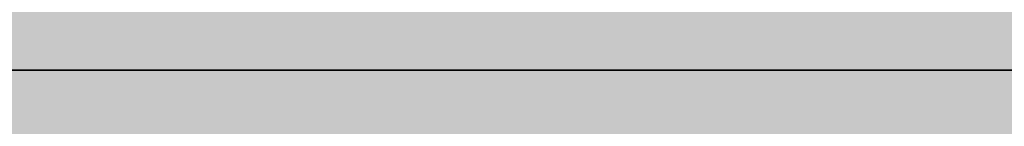
# Model space of a CAD drawing. Units: millimetres. Extents: x -22994 to 29398, y -19990 to 20176.
# Tile 76 of 135: x 226.355 to 227.437, y 84.498 to 84.615. Entities that reach past the tile are written whole.
import ezdxf
from ezdxf import colors
from ezdxf.entities.mleader import LeaderData, LeaderLine
from ezdxf.math import Vec2, Vec3

# ---------------------------------------------------------------- set-up
doc = ezdxf.new("R2010")
doc.units = ezdxf.units.MM
doc.header["$MEASUREMENT"] = 0
for name, color, linetype, lineweight in [('M-ANNO-TEXT', 7, 'Continuous', 25), ('M-DIMS', 2, 'Continuous', 18), ('M-EQPM-PATT', 7, 'Continuous', 18), ('M-PIPE', 7, 'Continuous', 35)]:
    doc.layers.add(name, color=color, linetype=linetype, lineweight=lineweight)
doc.styles.get("Standard").update_dxf_attribs({"font": 'arial.ttf'})
doc.dimstyles.get("Standard").update_dxf_attribs({"dimtxt": 0.18, "dimasz": 10000, "dimexe": 0.18, "dimexo": 0.0625, "dimgap": 0.09, "dimtad": 0, "dimtih": 1, "dimtoh": 1, "dimdec": 0, "dimzin": 0, "dimdsep": 46, "dimtxsty": 'Standard', "dimcen": 0.09, "dimadec": 0, "dimazin": 0, "dimtfac": 1, "dimtdec": 0, "dimtofl": 0, "dimtmove": 0, "dimatfit": 3, "dimfxl": 1, "dimtolj": 1, "dimtzin": 0, "dimlwd": 30, "dimarcsym": 0})

# ---------------------------------------------------------------- blocks, each defined once
blk = doc.blocks.new('*D2')
at = {"layer": 'Defpoints', "color": 0, "transparency": 16777216}
for p in [(6.6773, 10.2713), (290.852, 10.2713), (290.852, -5.0787)]:
    blk.add_point(p, dxfattribs=at)
at = {"layer": 'M-DIMS', "color": 0, "lineweight": -2, "transparency": 16777216}
for p, q in [((6.6773, 10.2088), (6.6773, -5.2587)), ((290.852, 10.2088), (290.852, -5.2587))]:
    blk.add_line(p, q, dxfattribs=at)
at = {"layer": 'M-DIMS', "color": 0, "lineweight": 30, "transparency": 16777216}
for p, q in [((-9993.3227, -5.0787), (-19993.3227, -5.0787)), ((10290.852, -5.0787), (20290.852, -5.0787))]:
    blk.add_line(p, q, dxfattribs=at)
at = {"layer": 'M-DIMS', "color": 0, "transparency": 16777216}
for points in [[(-9993.3227, 1661.5879), (-9993.3227, -1671.7454), (6.6773, -5.0787)], [(10290.852, 1661.5879), (10290.852, -1671.7454), (290.852, -5.0787)]]:
    blk.add_solid(points, dxfattribs=at)
at = {"layer": 'M-DIMS', "color": 0, "transparency": 16777216, "insert": (148.7647, -5.0787), "char_height": 0.18, "attachment_point": 5}
blk.add_mtext('\\A1;284.2', dxfattribs=at)
blk = doc.blocks.new('*D3')
at = {"layer": 'Defpoints', "color": 0, "transparency": 16777216}
for p in [(110.2647, 204.1654), (110.2647, 176.3662), (95.8327, 127.967)]:
    blk.add_point(p, dxfattribs=at)
at = {"layer": 'M-DIMS', "color": 0, "lineweight": -2, "transparency": 16777216}
for p, q in [((95.8327, 128.0295), (95.8327, 204.3454)), ((110.2647, 176.4287), (110.2647, 204.3454))]:
    blk.add_line(p, q, dxfattribs=at)
at = {"layer": 'M-DIMS', "color": 0, "lineweight": 30, "transparency": 16777216}
for p, q in [((-9904.1673, 204.1654), (-19904.1673, 204.1654)), ((10110.2647, 204.1654), (20110.2647, 204.1654))]:
    blk.add_line(p, q, dxfattribs=at)
at = {"layer": 'M-DIMS', "color": 0, "transparency": 16777216}
for points in [[(-9904.1673, 1870.8321), (-9904.1673, -1462.5013), (95.8327, 204.1654)], [(10110.2647, 1870.8321), (10110.2647, -1462.5013), (110.2647, 204.1654)]]:
    blk.add_solid(points, dxfattribs=at)
at = {"layer": 'M-DIMS', "color": 0, "transparency": 16777216, "insert": (103.0487, 204.1654), "char_height": 0.18, "attachment_point": 5}
blk.add_mtext('\\A1;14.432', dxfattribs=at)
blk = doc.blocks.new('*D4')
at = {"layer": 'Defpoints', "color": 0, "transparency": 16777216}
for p in [(116.2647, 204.1654), (110.2647, 176.3662), (116.2647, 176.3662)]:
    blk.add_point(p, dxfattribs=at)
at = {"layer": 'M-DIMS', "color": 0, "lineweight": -2, "transparency": 16777216}
for p, q in [((110.2647, 176.4287), (110.2647, 204.3454)), ((116.2647, 176.4287), (116.2647, 204.3454))]:
    blk.add_line(p, q, dxfattribs=at)
at = {"layer": 'M-DIMS', "color": 0, "lineweight": 30, "transparency": 16777216}
for p, q in [((-9889.7353, 204.1654), (-19889.7353, 204.1654)), ((10116.2647, 204.1654), (20116.2647, 204.1654))]:
    blk.add_line(p, q, dxfattribs=at)
at = {"layer": 'M-DIMS', "color": 0, "transparency": 16777216}
for points in [[(-9889.7353, 1870.8321), (-9889.7353, -1462.5013), (110.2647, 204.1654)], [(10116.2647, 1870.8321), (10116.2647, -1462.5013), (116.2647, 204.1654)]]:
    blk.add_solid(points, dxfattribs=at)
at = {"layer": 'M-DIMS', "color": 0, "transparency": 16777216, "insert": (113.2647, 204.1654), "char_height": 0.18, "attachment_point": 5}
blk.add_mtext('\\A1;6', dxfattribs=at)
blk = doc.blocks.new('*D5')
at = {"layer": 'Defpoints', "color": 0, "transparency": 16777216}
for p in [(181.2647, 204.1654), (116.2647, 176.3662), (181.2647, 176.3662)]:
    blk.add_point(p, dxfattribs=at)
at = {"layer": 'M-DIMS', "color": 0, "lineweight": -2, "transparency": 16777216}
for p, q in [((116.2647, 176.4287), (116.2647, 204.3454)), ((181.2647, 176.4287), (181.2647, 204.3454))]:
    blk.add_line(p, q, dxfattribs=at)
at = {"layer": 'M-DIMS', "color": 0, "lineweight": 30, "transparency": 16777216}
for p, q in [((-9883.7353, 204.1654), (-19883.7353, 204.1654)), ((10181.2647, 204.1654), (20181.2647, 204.1654))]:
    blk.add_line(p, q, dxfattribs=at)
at = {"layer": 'M-DIMS', "color": 0, "transparency": 16777216}
for points in [[(-9883.7353, 1870.8321), (-9883.7353, -1462.5013), (116.2647, 204.1654)], [(10181.2647, 1870.8321), (10181.2647, -1462.5013), (181.2647, 204.1654)]]:
    blk.add_solid(points, dxfattribs=at)
at = {"layer": 'M-DIMS', "color": 0, "transparency": 16777216, "insert": (148.7647, 204.1654), "char_height": 0.18, "attachment_point": 5}
blk.add_mtext('\\A1;65', dxfattribs=at)
blk = doc.blocks.new('*D6')
at = {"layer": 'Defpoints', "color": 0, "transparency": 16777216}
for p in [(187.2647, 204.1654), (181.2647, 176.3662), (187.2647, 176.3662)]:
    blk.add_point(p, dxfattribs=at)
at = {"layer": 'M-DIMS', "color": 0, "lineweight": -2, "transparency": 16777216}
for p, q in [((181.2647, 176.4287), (181.2647, 204.3454)), ((187.2647, 176.4287), (187.2647, 204.3454))]:
    blk.add_line(p, q, dxfattribs=at)
at = {"layer": 'M-DIMS', "color": 0, "lineweight": 30, "transparency": 16777216}
for p, q in [((-9818.7353, 204.1654), (-19818.7353, 204.1654)), ((10187.2647, 204.1654), (20187.2647, 204.1654))]:
    blk.add_line(p, q, dxfattribs=at)
at = {"layer": 'M-DIMS', "color": 0, "transparency": 16777216}
for points in [[(-9818.7353, 1870.8321), (-9818.7353, -1462.5013), (181.2647, 204.1654)], [(10187.2647, 1870.8321), (10187.2647, -1462.5013), (187.2647, 204.1654)]]:
    blk.add_solid(points, dxfattribs=at)
at = {"layer": 'M-DIMS', "color": 0, "transparency": 16777216, "insert": (184.2647, 204.1654), "char_height": 0.18, "attachment_point": 5}
blk.add_mtext('\\A1;6', dxfattribs=at)
blk = doc.blocks.new('*D7')
at = {"layer": 'Defpoints', "color": 0, "transparency": 16777216}
for p in [(201.6967, 204.1654), (187.2647, 176.3662), (201.6967, 127.967)]:
    blk.add_point(p, dxfattribs=at)
at = {"layer": 'M-DIMS', "color": 0, "lineweight": -2, "transparency": 16777216}
for p, q in [((187.2647, 176.4287), (187.2647, 204.3454)), ((201.6967, 128.0295), (201.6967, 204.3454))]:
    blk.add_line(p, q, dxfattribs=at)
at = {"layer": 'M-DIMS', "color": 0, "lineweight": 30, "transparency": 16777216}
for p, q in [((-9812.7353, 204.1654), (-19812.7353, 204.1654)), ((10201.6967, 204.1654), (20201.6967, 204.1654))]:
    blk.add_line(p, q, dxfattribs=at)
at = {"layer": 'M-DIMS', "color": 0, "transparency": 16777216}
for points in [[(-9812.7353, 1870.8321), (-9812.7353, -1462.5013), (187.2647, 204.1654)], [(10201.6967, 1870.8321), (10201.6967, -1462.5013), (201.6967, 204.1654)]]:
    blk.add_solid(points, dxfattribs=at)
at = {"layer": 'M-DIMS', "color": 0, "transparency": 16777216, "insert": (194.4807, 204.1654), "char_height": 0.18, "attachment_point": 5}
blk.add_mtext('\\A1;14.432', dxfattribs=at)
blk = doc.blocks.new('*D8')
at = {"layer": 'Defpoints', "color": 0, "transparency": 16777216}
for p in [(227.6485, 204.1654), (227.6485, 146.7296), (201.6967, 127.967)]:
    blk.add_point(p, dxfattribs=at)
at = {"layer": 'M-DIMS', "color": 0, "lineweight": -2, "transparency": 16777216}
for p, q in [((201.6967, 128.0295), (201.6967, 204.3454)), ((227.6485, 146.7921), (227.6485, 204.3454))]:
    blk.add_line(p, q, dxfattribs=at)
at = {"layer": 'M-DIMS', "color": 0, "lineweight": 30, "transparency": 16777216}
for p, q in [((-9798.3033, 204.1654), (-19798.3033, 204.1654)), ((10227.6485, 204.1654), (20227.6485, 204.1654))]:
    blk.add_line(p, q, dxfattribs=at)
at = {"layer": 'M-DIMS', "color": 0, "transparency": 16777216}
for points in [[(-9798.3033, 1870.8321), (-9798.3033, -1462.5013), (201.6967, 204.1654)], [(10227.6485, 1870.8321), (10227.6485, -1462.5013), (227.6485, 204.1654)]]:
    blk.add_solid(points, dxfattribs=at)
at = {"layer": 'M-DIMS', "color": 0, "transparency": 16777216, "insert": (214.6726, 204.1654), "char_height": 0.18, "attachment_point": 5}
blk.add_mtext('\\A1;25.95', dxfattribs=at)
blk = doc.blocks.new('*D9')
at = {"layer": 'Defpoints', "color": 0, "transparency": 16777216}
for p in [(187.2647, 176.3662), (306.202, 176.3662), (290.852, 10.2713)]:
    blk.add_point(p, dxfattribs=at)
at = {"layer": 'M-DIMS', "color": 0, "lineweight": 30, "transparency": 16777216}
for p, q in [((306.202, 10176.3662), (306.202, 20176.3662)), ((306.202, -9989.7287), (306.202, -19989.7287))]:
    blk.add_line(p, q, dxfattribs=at)
at = {"layer": 'M-DIMS', "color": 0, "lineweight": -2, "transparency": 16777216}
for p, q in [((187.3272, 176.3662), (306.382, 176.3662)), ((290.9145, 10.2713), (306.382, 10.2713))]:
    blk.add_line(p, q, dxfattribs=at)
at = {"layer": 'M-DIMS', "color": 0, "transparency": 16777216}
for points in [[(-1360.4646, 10176.3662), (1972.8687, 10176.3662), (306.202, 176.3662)], [(-1360.4646, -9989.7287), (1972.8687, -9989.7287), (306.202, 10.2713)]]:
    blk.add_solid(points, dxfattribs=at)
at = {"layer": 'M-DIMS', "color": 0, "transparency": 16777216, "insert": (306.202, 93.3187), "char_height": 0.18, "attachment_point": 5}
blk.add_mtext('\\A1;166.1', dxfattribs=at)
blk = doc.blocks.new('*D10')
at = {"layer": 'Defpoints', "color": 0, "transparency": 16777216}
for p in [(125.6498, 136.0713), (133.3459, 136.0713), (133.3459, -5.0787)]:
    blk.add_point(p, dxfattribs=at)
at = {"layer": 'M-DIMS', "color": 0, "lineweight": -2, "transparency": 16777216}
for p, q in [((125.6498, 136.0088), (125.6498, -5.2587)), ((133.3459, 136.0088), (133.3459, -5.2587))]:
    blk.add_line(p, q, dxfattribs=at)
at = {"layer": 'M-DIMS', "color": 0, "lineweight": 30, "transparency": 16777216}
for p, q in [((-9874.3502, -5.0787), (-19874.3502, -5.0787)), ((10133.3459, -5.0787), (20133.3459, -5.0787))]:
    blk.add_line(p, q, dxfattribs=at)
at = {"layer": 'M-DIMS', "color": 0, "transparency": 16777216}
for points in [[(-9874.3502, 1661.5879), (-9874.3502, -1671.7454), (125.6498, -5.0787)], [(10133.3459, 1661.5879), (10133.3459, -1671.7454), (133.3459, -5.0787)]]:
    blk.add_solid(points, dxfattribs=at)
at = {"layer": 'M-DIMS', "color": 0, "transparency": 16777216, "insert": (129.4978, -5.0787), "char_height": 0.18, "attachment_point": 5}
blk.add_mtext('\\A1;7.696', dxfattribs=at)
blk = doc.blocks.new('*D11')
at = {"layer": 'Defpoints', "color": 0, "transparency": 16777216}
for p in [(133.3459, 136.0713), (135.6498, 136.0713), (135.6498, -5.0787)]:
    blk.add_point(p, dxfattribs=at)
at = {"layer": 'M-DIMS', "color": 0, "lineweight": -2, "transparency": 16777216}
for p, q in [((133.3459, 136.0088), (133.3459, -5.2587)), ((135.6498, 136.0088), (135.6498, -5.2587))]:
    blk.add_line(p, q, dxfattribs=at)
at = {"layer": 'M-DIMS', "color": 0, "lineweight": 30, "transparency": 16777216}
for p, q in [((-9866.6541, -5.0787), (-19866.6541, -5.0787)), ((10135.6498, -5.0787), (20135.6498, -5.0787))]:
    blk.add_line(p, q, dxfattribs=at)
at = {"layer": 'M-DIMS', "color": 0, "transparency": 16777216}
for points in [[(-9866.6541, 1661.5879), (-9866.6541, -1671.7454), (133.3459, -5.0787)], [(10135.6498, 1661.5879), (10135.6498, -1671.7454), (135.6498, -5.0787)]]:
    blk.add_solid(points, dxfattribs=at)
at = {"layer": 'M-DIMS', "color": 0, "transparency": 16777216, "insert": (134.4978, -5.0787), "char_height": 0.18, "attachment_point": 5}
blk.add_mtext('\\A1;2.304', dxfattribs=at)
blk = doc.blocks.new('*D12')
at = {"layer": 'Defpoints', "color": 0, "transparency": 16777216}
for p in [(135.6498, 136.0713), (145.6498, 136.0713), (145.6498, -5.0787)]:
    blk.add_point(p, dxfattribs=at)
at = {"layer": 'M-DIMS', "color": 0, "lineweight": -2, "transparency": 16777216}
for p, q in [((135.6498, 136.0088), (135.6498, -5.2587)), ((145.6498, 136.0088), (145.6498, -5.2587))]:
    blk.add_line(p, q, dxfattribs=at)
at = {"layer": 'M-DIMS', "color": 0, "lineweight": 30, "transparency": 16777216}
for p, q in [((-9864.3502, -5.0787), (-19864.3502, -5.0787)), ((10145.6498, -5.0787), (20145.6498, -5.0787))]:
    blk.add_line(p, q, dxfattribs=at)
at = {"layer": 'M-DIMS', "color": 0, "transparency": 16777216}
for points in [[(-9864.3502, 1661.5879), (-9864.3502, -1671.7454), (135.6498, -5.0787)], [(10145.6498, 1661.5879), (10145.6498, -1671.7454), (145.6498, -5.0787)]]:
    blk.add_solid(points, dxfattribs=at)
at = {"layer": 'M-DIMS', "color": 0, "transparency": 16777216, "insert": (140.6498, -5.0787), "char_height": 0.18, "attachment_point": 5}
blk.add_mtext('\\A1;10', dxfattribs=at)
blk = doc.blocks.new('*D13')
at = {"layer": 'Defpoints', "color": 0, "transparency": 16777216}
for p in [(145.6498, 136.0713), (155.6498, 136.0713), (155.6498, -5.0787)]:
    blk.add_point(p, dxfattribs=at)
at = {"layer": 'M-DIMS', "color": 0, "lineweight": -2, "transparency": 16777216}
for p, q in [((145.6498, 136.0088), (145.6498, -5.2587)), ((155.6498, 136.0088), (155.6498, -5.2587))]:
    blk.add_line(p, q, dxfattribs=at)
at = {"layer": 'M-DIMS', "color": 0, "lineweight": 30, "transparency": 16777216}
for p, q in [((-9854.3502, -5.0787), (-19854.3502, -5.0787)), ((10155.6498, -5.0787), (20155.6498, -5.0787))]:
    blk.add_line(p, q, dxfattribs=at)
at = {"layer": 'M-DIMS', "color": 0, "transparency": 16777216}
for points in [[(-9854.3502, 1661.5879), (-9854.3502, -1671.7454), (145.6498, -5.0787)], [(10155.6498, 1661.5879), (10155.6498, -1671.7454), (155.6498, -5.0787)]]:
    blk.add_solid(points, dxfattribs=at)
at = {"layer": 'M-DIMS', "color": 0, "transparency": 16777216, "insert": (150.6498, -5.0787), "char_height": 0.18, "attachment_point": 5}
blk.add_mtext('\\A1;10', dxfattribs=at)
blk = doc.blocks.new('*D14')
at = {"layer": 'Defpoints', "color": 0, "transparency": 16777216}
for p in [(155.6498, 136.0713), (165.6498, 136.0713), (165.6498, -5.0787)]:
    blk.add_point(p, dxfattribs=at)
at = {"layer": 'M-DIMS', "color": 0, "lineweight": -2, "transparency": 16777216}
for p, q in [((155.6498, 136.0088), (155.6498, -5.2587)), ((165.6498, 136.0088), (165.6498, -5.2587))]:
    blk.add_line(p, q, dxfattribs=at)
at = {"layer": 'M-DIMS', "color": 0, "lineweight": 30, "transparency": 16777216}
for p, q in [((-9844.3502, -5.0787), (-19844.3502, -5.0787)), ((10165.6498, -5.0787), (20165.6498, -5.0787))]:
    blk.add_line(p, q, dxfattribs=at)
at = {"layer": 'M-DIMS', "color": 0, "transparency": 16777216}
for points in [[(-9844.3502, 1661.5879), (-9844.3502, -1671.7454), (155.6498, -5.0787)], [(10165.6498, 1661.5879), (10165.6498, -1671.7454), (165.6498, -5.0787)]]:
    blk.add_solid(points, dxfattribs=at)
at = {"layer": 'M-DIMS', "color": 0, "transparency": 16777216, "insert": (160.6498, -5.0787), "char_height": 0.18, "attachment_point": 5}
blk.add_mtext('\\A1;10', dxfattribs=at)
blk = doc.blocks.new('*D15')
at = {"layer": 'Defpoints', "color": 0, "transparency": 16777216}
for p in [(173.3459, 154.788), (173.3459, 136.0713), (306.202, 136.0713)]:
    blk.add_point(p, dxfattribs=at)
at = {"layer": 'M-DIMS', "color": 0, "lineweight": 30, "transparency": 16777216}
for p, q in [((306.202, 10154.788), (306.202, 20154.788)), ((306.202, -9863.9287), (306.202, -19863.9287))]:
    blk.add_line(p, q, dxfattribs=at)
at = {"layer": 'M-DIMS', "color": 0, "lineweight": -2, "transparency": 16777216}
for p, q in [((173.4084, 154.788), (306.382, 154.788)), ((173.4084, 136.0713), (306.382, 136.0713))]:
    blk.add_line(p, q, dxfattribs=at)
at = {"layer": 'M-DIMS', "color": 0, "transparency": 16777216}
for points in [[(-1360.4646, 10154.788), (1972.8687, 10154.788), (306.202, 154.788)], [(-1360.4646, -9863.9287), (1972.8687, -9863.9287), (306.202, 136.0713)]]:
    blk.add_solid(points, dxfattribs=at)
at = {"layer": 'M-DIMS', "color": 0, "transparency": 16777216, "insert": (306.202, 145.4297), "char_height": 0.18, "attachment_point": 5}
blk.add_mtext('\\A1;18.717', dxfattribs=at)
blk = doc.blocks.new('*D16')
at = {"layer": 'Defpoints', "color": 0, "transparency": 16777216}
for p in [(120.1702, 204.1654), (110.4658, 48.0349), (120.1702, 48.0349)]:
    blk.add_point(p, dxfattribs=at)
at = {"layer": 'M-DIMS', "color": 0, "lineweight": -2, "transparency": 16777216}
for p, q in [((110.4658, 48.0974), (110.4658, 204.3454)), ((120.1702, 48.0974), (120.1702, 204.3454))]:
    blk.add_line(p, q, dxfattribs=at)
at = {"layer": 'M-DIMS', "color": 0, "lineweight": 30, "transparency": 16777216}
for p, q in [((-9889.5342, 204.1654), (-19889.5342, 204.1654)), ((10120.1702, 204.1654), (20120.1702, 204.1654))]:
    blk.add_line(p, q, dxfattribs=at)
at = {"layer": 'M-DIMS', "color": 0, "transparency": 16777216}
for points in [[(-9889.5342, 1870.8321), (-9889.5342, -1462.5013), (110.4658, 204.1654)], [(10120.1702, 1870.8321), (10120.1702, -1462.5013), (120.1702, 204.1654)]]:
    blk.add_solid(points, dxfattribs=at)
at = {"layer": 'M-DIMS', "color": 0, "transparency": 16777216, "insert": (115.318, 204.1654), "char_height": 0.18, "attachment_point": 5}
blk.add_mtext('\\A1;9.704', dxfattribs=at)
blk = doc.blocks.new('*D17')
at = {"layer": 'Defpoints', "color": 0, "transparency": 16777216}
for p in [(126.1702, 204.1654), (120.1702, 48.0349), (126.1702, 48.0349)]:
    blk.add_point(p, dxfattribs=at)
at = {"layer": 'M-DIMS', "color": 0, "lineweight": -2, "transparency": 16777216}
for p, q in [((120.1702, 48.0974), (120.1702, 204.3454)), ((126.1702, 48.0974), (126.1702, 204.3454))]:
    blk.add_line(p, q, dxfattribs=at)
at = {"layer": 'M-DIMS', "color": 0, "lineweight": 30, "transparency": 16777216}
for p, q in [((-9879.8298, 204.1654), (-19879.8298, 204.1654)), ((10126.1702, 204.1654), (20126.1702, 204.1654))]:
    blk.add_line(p, q, dxfattribs=at)
at = {"layer": 'M-DIMS', "color": 0, "transparency": 16777216}
for points in [[(-9879.8298, 1870.8321), (-9879.8298, -1462.5013), (120.1702, 204.1654)], [(10126.1702, 1870.8321), (10126.1702, -1462.5013), (126.1702, 204.1654)]]:
    blk.add_solid(points, dxfattribs=at)
at = {"layer": 'M-DIMS', "color": 0, "transparency": 16777216, "insert": (123.1702, 204.1654), "char_height": 0.18, "attachment_point": 5}
blk.add_mtext('\\A1;6', dxfattribs=at)
blk = doc.blocks.new('*D18')
at = {"layer": 'Defpoints', "color": 0, "transparency": 16777216}
for p in [(132.1702, 204.1654), (126.1702, 48.0349), (132.1702, 48.0349)]:
    blk.add_point(p, dxfattribs=at)
at = {"layer": 'M-DIMS', "color": 0, "lineweight": -2, "transparency": 16777216}
for p, q in [((126.1702, 48.0974), (126.1702, 204.3454)), ((132.1702, 48.0974), (132.1702, 204.3454))]:
    blk.add_line(p, q, dxfattribs=at)
at = {"layer": 'M-DIMS', "color": 0, "lineweight": 30, "transparency": 16777216}
for p, q in [((-9873.8298, 204.1654), (-19873.8298, 204.1654)), ((10132.1702, 204.1654), (20132.1702, 204.1654))]:
    blk.add_line(p, q, dxfattribs=at)
at = {"layer": 'M-DIMS', "color": 0, "transparency": 16777216}
for points in [[(-9873.8298, 1870.8321), (-9873.8298, -1462.5013), (126.1702, 204.1654)], [(10132.1702, 1870.8321), (10132.1702, -1462.5013), (132.1702, 204.1654)]]:
    blk.add_solid(points, dxfattribs=at)
at = {"layer": 'M-DIMS', "color": 0, "transparency": 16777216, "insert": (129.1702, 204.1654), "char_height": 0.18, "attachment_point": 5}
blk.add_mtext('\\A1;6', dxfattribs=at)
blk = doc.blocks.new('*D19')
at = {"layer": 'Defpoints', "color": 0, "transparency": 16777216}
for p in [(138.1702, 204.1654), (132.1702, 48.0349), (138.1702, 48.0349)]:
    blk.add_point(p, dxfattribs=at)
at = {"layer": 'M-DIMS', "color": 0, "lineweight": -2, "transparency": 16777216}
for p, q in [((132.1702, 48.0974), (132.1702, 204.3454)), ((138.1702, 48.0974), (138.1702, 204.3454))]:
    blk.add_line(p, q, dxfattribs=at)
at = {"layer": 'M-DIMS', "color": 0, "lineweight": 30, "transparency": 16777216}
for p, q in [((-9867.8298, 204.1654), (-19867.8298, 204.1654)), ((10138.1702, 204.1654), (20138.1702, 204.1654))]:
    blk.add_line(p, q, dxfattribs=at)
at = {"layer": 'M-DIMS', "color": 0, "transparency": 16777216}
for points in [[(-9867.8298, 1870.8321), (-9867.8298, -1462.5013), (132.1702, 204.1654)], [(10138.1702, 1870.8321), (10138.1702, -1462.5013), (138.1702, 204.1654)]]:
    blk.add_solid(points, dxfattribs=at)
at = {"layer": 'M-DIMS', "color": 0, "transparency": 16777216, "insert": (135.1702, 204.1654), "char_height": 0.18, "attachment_point": 5}
blk.add_mtext('\\A1;6', dxfattribs=at)
blk = doc.blocks.new('*D20')
at = {"layer": 'Defpoints', "color": 0, "transparency": 16777216}
for p in [(144.1702, 204.1654), (138.1702, 48.0349), (144.1702, 48.0349)]:
    blk.add_point(p, dxfattribs=at)
at = {"layer": 'M-DIMS', "color": 0, "lineweight": -2, "transparency": 16777216}
for p, q in [((138.1702, 48.0974), (138.1702, 204.3454)), ((144.1702, 48.0974), (144.1702, 204.3454))]:
    blk.add_line(p, q, dxfattribs=at)
at = {"layer": 'M-DIMS', "color": 0, "lineweight": 30, "transparency": 16777216}
for p, q in [((-9861.8298, 204.1654), (-19861.8298, 204.1654)), ((10144.1702, 204.1654), (20144.1702, 204.1654))]:
    blk.add_line(p, q, dxfattribs=at)
at = {"layer": 'M-DIMS', "color": 0, "transparency": 16777216}
for points in [[(-9861.8298, 1870.8321), (-9861.8298, -1462.5013), (138.1702, 204.1654)], [(10144.1702, 1870.8321), (10144.1702, -1462.5013), (144.1702, 204.1654)]]:
    blk.add_solid(points, dxfattribs=at)
at = {"layer": 'M-DIMS', "color": 0, "transparency": 16777216, "insert": (141.1702, 204.1654), "char_height": 0.18, "attachment_point": 5}
blk.add_mtext('\\A1;6', dxfattribs=at)
blk = doc.blocks.new('*D21')
at = {"layer": 'Defpoints', "color": 0, "transparency": 16777216}
for p in [(149.1157, 204.1654), (144.1702, 48.0349), (149.1157, 48.0349)]:
    blk.add_point(p, dxfattribs=at)
at = {"layer": 'M-DIMS', "color": 0, "lineweight": -2, "transparency": 16777216}
for p, q in [((144.1702, 48.0974), (144.1702, 204.3454)), ((149.1157, 48.0974), (149.1157, 204.3454))]:
    blk.add_line(p, q, dxfattribs=at)
at = {"layer": 'M-DIMS', "color": 0, "lineweight": 30, "transparency": 16777216}
for p, q in [((-9855.8298, 204.1654), (-19855.8298, 204.1654)), ((10149.1157, 204.1654), (20149.1157, 204.1654))]:
    blk.add_line(p, q, dxfattribs=at)
at = {"layer": 'M-DIMS', "color": 0, "transparency": 16777216}
for points in [[(-9855.8298, 1870.8321), (-9855.8298, -1462.5013), (144.1702, 204.1654)], [(10149.1157, 1870.8321), (10149.1157, -1462.5013), (149.1157, 204.1654)]]:
    blk.add_solid(points, dxfattribs=at)
at = {"layer": 'M-DIMS', "color": 0, "transparency": 16777216, "insert": (146.6429, 204.1654), "char_height": 0.18, "attachment_point": 5}
blk.add_mtext('\\A1;4.945', dxfattribs=at)
blk = doc.blocks.new('*D22')
at = {"layer": 'Defpoints', "color": 0, "transparency": 16777216}
for p in [(149.1157, 30.9895), (155.1157, 30.9895), (155.1157, -5.0787)]:
    blk.add_point(p, dxfattribs=at)
at = {"layer": 'M-DIMS', "color": 0, "lineweight": -2, "transparency": 16777216}
for p, q in [((149.1157, 30.927), (149.1157, -5.2587)), ((155.1157, 30.927), (155.1157, -5.2587))]:
    blk.add_line(p, q, dxfattribs=at)
at = {"layer": 'M-DIMS', "color": 0, "lineweight": 30, "transparency": 16777216}
for p, q in [((-9850.8843, -5.0787), (-19850.8843, -5.0787)), ((10155.1157, -5.0787), (20155.1157, -5.0787))]:
    blk.add_line(p, q, dxfattribs=at)
at = {"layer": 'M-DIMS', "color": 0, "transparency": 16777216}
for points in [[(-9850.8843, 1661.5879), (-9850.8843, -1671.7454), (149.1157, -5.0787)], [(10155.1157, 1661.5879), (10155.1157, -1671.7454), (155.1157, -5.0787)]]:
    blk.add_solid(points, dxfattribs=at)
at = {"layer": 'M-DIMS', "color": 0, "transparency": 16777216, "insert": (152.1157, -5.0787), "char_height": 0.18, "attachment_point": 5}
blk.add_mtext('\\A1;6', dxfattribs=at)
blk = doc.blocks.new('*D23')
at = {"layer": 'Defpoints', "color": 0, "transparency": 16777216}
for p in [(155.1157, 30.9895), (161.1157, 30.9895), (161.1157, -5.0787)]:
    blk.add_point(p, dxfattribs=at)
at = {"layer": 'M-DIMS', "color": 0, "lineweight": -2, "transparency": 16777216}
for p, q in [((155.1157, 30.927), (155.1157, -5.2587)), ((161.1157, 30.927), (161.1157, -5.2587))]:
    blk.add_line(p, q, dxfattribs=at)
at = {"layer": 'M-DIMS', "color": 0, "lineweight": 30, "transparency": 16777216}
for p, q in [((-9844.8843, -5.0787), (-19844.8843, -5.0787)), ((10161.1157, -5.0787), (20161.1157, -5.0787))]:
    blk.add_line(p, q, dxfattribs=at)
at = {"layer": 'M-DIMS', "color": 0, "transparency": 16777216}
for points in [[(-9844.8843, 1661.5879), (-9844.8843, -1671.7454), (155.1157, -5.0787)], [(10161.1157, 1661.5879), (10161.1157, -1671.7454), (161.1157, -5.0787)]]:
    blk.add_solid(points, dxfattribs=at)
at = {"layer": 'M-DIMS', "color": 0, "transparency": 16777216, "insert": (158.1157, -5.0787), "char_height": 0.18, "attachment_point": 5}
blk.add_mtext('\\A1;6', dxfattribs=at)
blk = doc.blocks.new('*D24')
at = {"layer": 'Defpoints', "color": 0, "transparency": 16777216}
for p in [(161.1157, 30.9895), (166.4387, 30.9895), (166.4387, -5.0787)]:
    blk.add_point(p, dxfattribs=at)
at = {"layer": 'M-DIMS', "color": 0, "lineweight": -2, "transparency": 16777216}
for p, q in [((161.1157, 30.927), (161.1157, -5.2587)), ((166.4387, 30.927), (166.4387, -5.2587))]:
    blk.add_line(p, q, dxfattribs=at)
at = {"layer": 'M-DIMS', "color": 0, "lineweight": 30, "transparency": 16777216}
for p, q in [((-9838.8843, -5.0787), (-19838.8843, -5.0787)), ((10166.4387, -5.0787), (20166.4387, -5.0787))]:
    blk.add_line(p, q, dxfattribs=at)
at = {"layer": 'M-DIMS', "color": 0, "transparency": 16777216}
for points in [[(-9838.8843, 1661.5879), (-9838.8843, -1671.7454), (161.1157, -5.0787)], [(10166.4387, 1661.5879), (10166.4387, -1671.7454), (166.4387, -5.0787)]]:
    blk.add_solid(points, dxfattribs=at)
at = {"layer": 'M-DIMS', "color": 0, "transparency": 16777216, "insert": (163.7772, -5.0787), "char_height": 0.18, "attachment_point": 5}
blk.add_mtext('\\A1;5.323', dxfattribs=at)
blk = doc.blocks.new('*D25')
at = {"layer": 'Defpoints', "color": 0, "transparency": 16777216}
for p in [(166.4387, 30.9895), (172.4387, 30.9895), (172.4387, -5.0787)]:
    blk.add_point(p, dxfattribs=at)
at = {"layer": 'M-DIMS', "color": 0, "lineweight": -2, "transparency": 16777216}
for p, q in [((166.4387, 30.927), (166.4387, -5.2587)), ((172.4387, 30.927), (172.4387, -5.2587))]:
    blk.add_line(p, q, dxfattribs=at)
at = {"layer": 'M-DIMS', "color": 0, "lineweight": 30, "transparency": 16777216}
for p, q in [((-9833.5613, -5.0787), (-19833.5613, -5.0787)), ((10172.4387, -5.0787), (20172.4387, -5.0787))]:
    blk.add_line(p, q, dxfattribs=at)
at = {"layer": 'M-DIMS', "color": 0, "transparency": 16777216}
for points in [[(-9833.5613, 1661.5879), (-9833.5613, -1671.7454), (166.4387, -5.0787)], [(10172.4387, 1661.5879), (10172.4387, -1671.7454), (172.4387, -5.0787)]]:
    blk.add_solid(points, dxfattribs=at)
at = {"layer": 'M-DIMS', "color": 0, "transparency": 16777216, "insert": (169.4387, -5.0787), "char_height": 0.18, "attachment_point": 5}
blk.add_mtext('\\A1;6', dxfattribs=at)
blk = doc.blocks.new('*D26')
at = {"layer": 'Defpoints', "color": 0, "transparency": 16777216}
for p in [(172.4387, 30.9895), (178.4387, 30.9895), (178.4387, -5.0787)]:
    blk.add_point(p, dxfattribs=at)
at = {"layer": 'M-DIMS', "color": 0, "lineweight": -2, "transparency": 16777216}
for p, q in [((172.4387, 30.927), (172.4387, -5.2587)), ((178.4387, 30.927), (178.4387, -5.2587))]:
    blk.add_line(p, q, dxfattribs=at)
at = {"layer": 'M-DIMS', "color": 0, "lineweight": 30, "transparency": 16777216}
for p, q in [((-9827.5613, -5.0787), (-19827.5613, -5.0787)), ((10178.4387, -5.0787), (20178.4387, -5.0787))]:
    blk.add_line(p, q, dxfattribs=at)
at = {"layer": 'M-DIMS', "color": 0, "transparency": 16777216}
for points in [[(-9827.5613, 1661.5879), (-9827.5613, -1671.7454), (172.4387, -5.0787)], [(10178.4387, 1661.5879), (10178.4387, -1671.7454), (178.4387, -5.0787)]]:
    blk.add_solid(points, dxfattribs=at)
at = {"layer": 'M-DIMS', "color": 0, "transparency": 16777216, "insert": (175.4387, -5.0787), "char_height": 0.18, "attachment_point": 5}
blk.add_mtext('\\A1;6', dxfattribs=at)
blk = doc.blocks.new('*D27')
at = {"layer": 'Defpoints', "color": 0, "transparency": 16777216}
for p in [(178.4387, 30.9895), (188.1175, 30.9895), (188.1175, -5.0787)]:
    blk.add_point(p, dxfattribs=at)
at = {"layer": 'M-DIMS', "color": 0, "lineweight": -2, "transparency": 16777216}
for p, q in [((178.4387, 30.927), (178.4387, -5.2587)), ((188.1175, 30.927), (188.1175, -5.2587))]:
    blk.add_line(p, q, dxfattribs=at)
at = {"layer": 'M-DIMS', "color": 0, "lineweight": 30, "transparency": 16777216}
for p, q in [((-9821.5613, -5.0787), (-19821.5613, -5.0787)), ((10188.1175, -5.0787), (20188.1175, -5.0787))]:
    blk.add_line(p, q, dxfattribs=at)
at = {"layer": 'M-DIMS', "color": 0, "transparency": 16777216}
for points in [[(-9821.5613, 1661.5879), (-9821.5613, -1671.7454), (178.4387, -5.0787)], [(10188.1175, 1661.5879), (10188.1175, -1671.7454), (188.1175, -5.0787)]]:
    blk.add_solid(points, dxfattribs=at)
at = {"layer": 'M-DIMS', "color": 0, "transparency": 16777216, "insert": (183.2781, -5.0787), "char_height": 0.18, "attachment_point": 5}
blk.add_mtext('\\A1;9.679', dxfattribs=at)
blk = doc.blocks.new('*D28')
at = {"layer": 'Defpoints', "color": 0, "transparency": 16777216}
for p in [(188.1175, 48.0349), (306.202, 48.0349), (188.1175, 30.9895)]:
    blk.add_point(p, dxfattribs=at)
at = {"layer": 'M-DIMS', "color": 0, "lineweight": 30, "transparency": 16777216}
for p, q in [((306.202, 10048.0349), (306.202, 20048.0349)), ((306.202, -9969.0105), (306.202, -19969.0105))]:
    blk.add_line(p, q, dxfattribs=at)
at = {"layer": 'M-DIMS', "color": 0, "lineweight": -2, "transparency": 16777216}
for p, q in [((188.18, 48.0349), (306.382, 48.0349)), ((188.18, 30.9895), (306.382, 30.9895))]:
    blk.add_line(p, q, dxfattribs=at)
at = {"layer": 'M-DIMS', "color": 0, "transparency": 16777216}
for points in [[(-1360.4646, 10048.0349), (1972.8687, 10048.0349), (306.202, 48.0349)], [(-1360.4646, -9969.0105), (1972.8687, -9969.0105), (306.202, 30.9895)]]:
    blk.add_solid(points, dxfattribs=at)
at = {"layer": 'M-DIMS', "color": 0, "transparency": 16777216, "insert": (306.202, 39.5122), "char_height": 0.18, "attachment_point": 5}
blk.add_mtext('\\A1;17.045', dxfattribs=at)
blk = doc.blocks.new('*D29')
at = {"layer": 'Defpoints', "color": 0, "transparency": 16777216}
for p in [(36.8006, 80.045), (64.0296, 80.045)]:
    blk.add_point(p, dxfattribs=at)
at = {"layer": 'M-DIMS', "color": 0, "lineweight": -2, "transparency": 16777216}
for p, q in [((50.4151, 79.955), (50.4151, 80.135)), ((50.3251, 80.045), (50.5051, 80.045))]:
    blk.add_line(p, q, dxfattribs=at)
at = {"layer": 'M-DIMS', "color": 0, "lineweight": 30, "transparency": 16777216}
blk.add_line((20064.0296, 80.0303), (10064.0296, 80.0377), dxfattribs=at)
at = {"layer": 'M-DIMS', "color": 0, "transparency": 16777216}
blk.add_solid([(10064.0309, 1746.7043), (10064.0284, -1586.629), (64.0296, 80.045)], dxfattribs=at)
at = {"layer": 'M-DIMS', "color": 0, "transparency": 16777216, "insert": (20064.5213, 80.0303), "char_height": 0.18, "attachment_point": 5}
blk.add_mtext('\\A1;∅27.23', dxfattribs=at)
blk = doc.blocks.new('*D30')
at = {"layer": 'Defpoints', "color": 0, "transparency": 16777216}
for p in [(216.3148, 146.7291), (238.9821, 146.73)]:
    blk.add_point(p, dxfattribs=at)
at = {"layer": 'M-DIMS', "color": 0, "lineweight": 30, "transparency": 16777216}
blk.add_line((20238.9821, 147.4959), (10238.9821, 147.1129), dxfattribs=at)
at = {"layer": 'M-DIMS', "color": 0, "lineweight": -2, "transparency": 16777216}
for p, q in [((227.6485, 146.6396), (227.6485, 146.8196)), ((227.5585, 146.7296), (227.7385, 146.7296))]:
    blk.add_line(p, q, dxfattribs=at)
at = {"layer": 'M-DIMS', "color": 0, "transparency": 16777216}
blk.add_solid([(10238.9183, 1813.7796), (10239.0459, -1519.5537), (238.9821, 146.73)], dxfattribs=at)
at = {"layer": 'M-DIMS', "color": 0, "transparency": 16777216, "insert": (20239.5436, 147.4959), "char_height": 0.18, "attachment_point": 5}
blk.add_mtext('\\A1;∅22.667', dxfattribs=at)
blk = doc.blocks.new('*D31')
at = {"layer": 'Defpoints', "color": 0, "transparency": 16777216}
for p in [(223.1641, 146.7291), (232.1328, 146.73)]:
    blk.add_point(p, dxfattribs=at)
at = {"layer": 'M-DIMS', "color": 0, "lineweight": 30, "transparency": 16777216}
blk.add_line((20232.1327, 148.6656), (10232.1328, 147.6978), dxfattribs=at)
at = {"layer": 'M-DIMS', "color": 0, "lineweight": -2, "transparency": 16777216}
for p, q in [((227.6485, 146.6396), (227.6485, 146.8196)), ((227.5585, 146.7296), (227.7385, 146.7296))]:
    blk.add_line(p, q, dxfattribs=at)
at = {"layer": 'M-DIMS', "color": 0, "transparency": 16777216}
blk.add_solid([(10231.9715, 1814.3645), (10232.2941, -1518.9688), (232.1328, 146.73)], dxfattribs=at)
at = {"layer": 'M-DIMS', "color": 0, "transparency": 16777216, "insert": (20232.6245, 148.6656), "char_height": 0.18, "attachment_point": 5}
blk.add_mtext('\\A1;∅8.969', dxfattribs=at)
blk = doc.blocks.new('*D36')
at = {"layer": 'Defpoints', "color": 0, "transparency": 16777216}
for p in [(46.39, 31.3035), (46.3875, 26.5934)]:
    blk.add_point(p, dxfattribs=at)
at = {"layer": 'M-DIMS', "color": 0, "lineweight": 30, "transparency": 16777216}
for p, q in [((57.1499, 20031.3006), (51.77, 10031.302)), ((10057.1499, 20031.3006), (57.1499, 20031.3006))]:
    blk.add_line(p, q, dxfattribs=at)
at = {"layer": 'M-DIMS', "color": 0, "lineweight": -2, "transparency": 16777216}
for p, q in [((46.3887, 28.8585), (46.3887, 29.0385)), ((46.2987, 28.9485), (46.4787, 28.9485))]:
    blk.add_line(p, q, dxfattribs=at)
at = {"layer": 'M-DIMS', "color": 0, "transparency": 16777216}
blk.add_solid([(-1614.8965, 10032.1987), (1718.4364, 10030.4054), (46.39, 31.3035)], dxfattribs=at)
at = {"layer": 'M-DIMS', "color": 0, "transparency": 16777216, "insert": (10057.5542, 20031.3006), "char_height": 0.18, "attachment_point": 5}
blk.add_mtext('\\A1;∅4.71', dxfattribs=at)
blk = doc.blocks.new('*D37')
at = {"layer": 'Defpoints', "color": 0, "transparency": 16777216}
for p in [(54.8343, 118.6145), (59.4936, 118.614)]:
    blk.add_point(p, dxfattribs=at)
at = {"layer": 'M-DIMS', "color": 0, "lineweight": -2, "transparency": 16777216}
for p, q in [((57.1639, 118.5243), (57.1639, 118.7043)), ((57.0739, 118.6143), (57.2539, 118.6143))]:
    blk.add_line(p, q, dxfattribs=at)
at = {"layer": 'M-DIMS', "color": 0, "lineweight": 30, "transparency": 16777216}
blk.add_line((20059.4934, 116.2531), (10059.4935, 117.4336), dxfattribs=at)
at = {"layer": 'M-DIMS', "color": 0, "transparency": 16777216}
blk.add_solid([(10059.6902, 1784.1002), (10059.2968, -1549.2331), (59.4936, 118.614)], dxfattribs=at)
at = {"layer": 'M-DIMS', "color": 0, "transparency": 16777216, "insert": (20059.9852, 116.2531), "char_height": 0.18, "attachment_point": 5}
blk.add_mtext('\\A1;∅4.659', dxfattribs=at)

msp = doc.modelspace()

# ---------------------------------------------------------------- hatches: boundary and pattern name
at = {"layer": 'M-EQPM-PATT'}
h = msp.add_hatch(color=256, dxfattribs=at)
h.set_gradient(color1=(205, 32, 39), color2=(205, 32, 39), tint=1)
h.paths.add_polyline_path([(116.2647, 150.3662), (116.2647, 170.3662), (116.2647, 176.3662), (110.2647, 176.3662), (110.2647, 152.0276), (95.8327, 127.967), (95.8327, 16.6063), (201.6967, 16.6063), (201.6967, 127.967), (187.2647, 152.0276), (187.2647, 176.3662), (181.2647, 176.3662), (181.2647, 170.3662), (181.2647, 150.3662), (195.6967, 126.3055), (195.6967, 22.6063), (101.8327, 22.6063), (101.8327, 126.3055)])
h.paths.add_polyline_path([(185.2208, 88.6347), (101.8327, 88.6347), (101.8327, 87.6347), (182.8066, 87.6347), (178.7313, 83.5594), (195.6967, 83.5594), (195.6967, 84.5594), (181.1455, 84.5594)], flags=17)
h.paths.add_polyline_path([(95.8327, 88.6347), (60.9779, 88.6347, -0.022855), (61.7178, 87.6347), (95.8327, 87.6347)])
h.paths.add_polyline_path([(215.6212, 86.5189), (215.6212, 80.5999), (220.5095, 83.5594)])
h.paths.add_polyline_path([(215.6212, 84.5594), (201.6967, 84.5594), (201.6967, 83.5594), (215.6212, 83.5594)])
h.paths.add_polyline_path([(225.3978, 86.5189), (220.5095, 83.5594), (225.3978, 80.5999)])
h.paths.add_polyline_path([(231.6256, 84.5594), (225.3978, 84.5594), (225.3978, 83.5594), (231.6256, 83.5594)])

# ---------------------------------------------------------------- linework, layer by layer
at = {"layer": 'M-PIPE'}
msp.add_line((225.3978, 84.5594), (231.6256, 84.5594), dxfattribs=at)

# ---------------------------------------------------------------- dimensions: what is measured, and where the dimension line sits
at = {"layer": 'M-DIMS'}
for base, p1, p2, override, picture, middle in [((306.202, 176.3662), (290.852, 10.2713), (187.2647, 176.3662), {"dimdec": 1, "dimlfac": 1, "dimrnd": 0, "dimzin": 0, "dimdsep": 46, "dimlunit": 2}, '*D9', (306.202, 93.3187)), ((306.202, 136.0713), (173.3459, 154.788), (173.3459, 136.0713), {"dimdec": 3, "dimlfac": 1, "dimrnd": 0, "dimzin": 0, "dimdsep": 46, "dimlunit": 2}, '*D15', (306.202, 145.4297)), ((306.202, 48.0349), (188.1175, 30.9895), (188.1175, 48.0349), {"dimdec": 3, "dimlfac": 1, "dimrnd": 0, "dimzin": 0, "dimdsep": 46, "dimlunit": 2}, '*D28', (306.202, 39.5122))]:
    dim = msp.add_linear_dim(base=base, p1=p1, p2=p2, angle=90, dimstyle='Standard', override=override, dxfattribs=at)
    dim.commit()
    dim.dimension.update_dxf_attribs({"geometry": picture, "text_midpoint": middle})
for p1, p2, override, picture, middle in [((46.3875, 26.5934), (46.39, 31.3035), {"dimdec": 2, "dimlfac": 1, "dimrnd": 0, "dimzin": 0, "dimdsep": 46, "dimlunit": 2}, '*D36', (10057.5542, 20031.3006)), ((223.1641, 146.7291), (232.1328, 146.73), {"dimdec": 3, "dimlfac": 1, "dimrnd": 0, "dimzin": 0, "dimdsep": 46, "dimlunit": 2}, '*D31', (20232.1327, 148.6656)), ((216.3148, 146.7291), (238.9821, 146.73), {"dimdec": 3, "dimlfac": 1, "dimrnd": 0, "dimzin": 0, "dimdsep": 46, "dimlunit": 2}, '*D30', (20238.9821, 147.4959))]:
    dim = msp.add_diameter_dim_2p(p1=p1, p2=p2, dimstyle='Standard', override=override, dxfattribs=at)
    dim.commit()
    dim.dimension.update_dxf_attribs({"geometry": picture, "text_midpoint": middle, "dimtype": 163})
for base, p1, p2, override, picture, middle in [((110.2647, 204.1654), (95.8327, 127.967), (110.2647, 176.3662), {"dimdec": 3, "dimlfac": 1, "dimrnd": 0, "dimzin": 0, "dimdsep": 46, "dimlunit": 2}, '*D3', (103.0487, 204.1654)), ((116.2647, 204.1654), (110.2647, 176.3662), (116.2647, 176.3662), {"dimdec": 0, "dimlfac": 1, "dimrnd": 0, "dimzin": 0, "dimdsep": 46, "dimlunit": 2}, '*D4', (113.2647, 204.1654)), ((120.1702, 204.1654), (110.4658, 48.0349), (120.1702, 48.0349), {"dimdec": 3, "dimlfac": 1, "dimrnd": 0, "dimzin": 0, "dimdsep": 46, "dimlunit": 2}, '*D16', (115.318, 204.1654)), ((181.2647, 204.1654), (116.2647, 176.3662), (181.2647, 176.3662), {"dimdec": 0, "dimlfac": 1, "dimrnd": 0, "dimzin": 0, "dimdsep": 46, "dimlunit": 2}, '*D5', (148.7647, 204.1654)), ((126.1702, 204.1654), (120.1702, 48.0349), (126.1702, 48.0349), {"dimdec": 0, "dimlfac": 1, "dimrnd": 0, "dimzin": 0, "dimdsep": 46, "dimlunit": 2}, '*D17', (123.1702, 204.1654)), ((132.1702, 204.1654), (126.1702, 48.0349), (132.1702, 48.0349), {"dimdec": 0, "dimlfac": 1, "dimrnd": 0, "dimzin": 0, "dimdsep": 46, "dimlunit": 2}, '*D18', (129.1702, 204.1654)), ((138.1702, 204.1654), (132.1702, 48.0349), (138.1702, 48.0349), {"dimdec": 0, "dimlfac": 1, "dimrnd": 0, "dimzin": 0, "dimdsep": 46, "dimlunit": 2}, '*D19', (135.1702, 204.1654)), ((144.1702, 204.1654), (138.1702, 48.0349), (144.1702, 48.0349), {"dimdec": 0, "dimlfac": 1, "dimrnd": 0, "dimzin": 0, "dimdsep": 46, "dimlunit": 2}, '*D20', (141.1702, 204.1654)), ((149.11567, 204.16539), (144.17023, 48.03494), (149.11567, 48.03494), {"dimdec": 3, "dimlfac": 1, "dimrnd": 0, "dimzin": 0, "dimdsep": 46, "dimlunit": 2}, '*D21', (146.64295, 204.16539)), ((187.2647, 204.1654), (181.2647, 176.3662), (187.2647, 176.3662), {"dimdec": 0, "dimlfac": 1, "dimrnd": 0, "dimzin": 0, "dimdsep": 46, "dimlunit": 2}, '*D6', (184.2647, 204.1654)), ((201.6967, 204.1654), (187.2647, 176.3662), (201.6967, 127.967), {"dimdec": 3, "dimlfac": 1, "dimrnd": 0, "dimzin": 0, "dimdsep": 46, "dimlunit": 2}, '*D7', (194.4807, 204.1654)), ((227.6485, 204.1654), (201.6967, 127.967), (227.6485, 146.7296), {"dimdec": 2, "dimlfac": 1, "dimrnd": 0, "dimzin": 0, "dimdsep": 46, "dimlunit": 2}, '*D8', (214.6726, 204.1654)), ((290.852, -5.0787), (6.6773, 10.2713), (290.852, 10.2713), {"dimdec": 1, "dimlfac": 1, "dimrnd": 0, "dimzin": 0, "dimdsep": 46, "dimlunit": 2}, '*D2', (148.7647, -5.0787)), ((133.3459, -5.0787), (125.6498, 136.0713), (133.3459, 136.0713), {"dimdec": 3, "dimlfac": 1, "dimrnd": 0, "dimzin": 0, "dimdsep": 46, "dimlunit": 2}, '*D10', (129.4978, -5.0787)), ((135.6498, -5.0787), (133.3459, 136.0713), (135.6498, 136.0713), {"dimdec": 3, "dimlfac": 1, "dimrnd": 0, "dimzin": 0, "dimdsep": 46, "dimlunit": 2}, '*D11', (134.4978, -5.0787)), ((145.6498, -5.0787), (135.6498, 136.0713), (145.6498, 136.0713), {"dimdec": 0, "dimlfac": 1, "dimrnd": 0, "dimzin": 0, "dimdsep": 46, "dimlunit": 2}, '*D12', (140.6498, -5.0787)), ((155.6498, -5.0787), (145.6498, 136.0713), (155.6498, 136.0713), {"dimdec": 0, "dimlfac": 1, "dimrnd": 0, "dimzin": 0, "dimdsep": 46, "dimlunit": 2}, '*D13', (150.6498, -5.0787)), ((155.1157, -5.0787), (149.1157, 30.9895), (155.1157, 30.9895), {"dimdec": 0, "dimlfac": 1, "dimrnd": 0, "dimzin": 0, "dimdsep": 46, "dimlunit": 2}, '*D22', (152.1157, -5.0787)), ((161.1157, -5.0787), (155.1157, 30.9895), (161.1157, 30.9895), {"dimdec": 0, "dimlfac": 1, "dimrnd": 0, "dimzin": 0, "dimdsep": 46, "dimlunit": 2}, '*D23', (158.1157, -5.0787)), ((165.6498, -5.0787), (155.6498, 136.0713), (165.6498, 136.0713), {"dimdec": 0, "dimlfac": 1, "dimrnd": 0, "dimzin": 0, "dimdsep": 46, "dimlunit": 2}, '*D14', (160.6498, -5.0787)), ((166.4387, -5.0787), (161.1157, 30.9895), (166.4387, 30.9895), {"dimdec": 3, "dimlfac": 1, "dimrnd": 0, "dimzin": 0, "dimdsep": 46, "dimlunit": 2}, '*D24', (163.7772, -5.0787)), ((172.4387, -5.0787), (166.4387, 30.9895), (172.4387, 30.9895), {"dimdec": 0, "dimlfac": 1, "dimrnd": 0, "dimzin": 0, "dimdsep": 46, "dimlunit": 2}, '*D25', (169.4387, -5.0787)), ((178.4387, -5.0787), (172.4387, 30.9895), (178.4387, 30.9895), {"dimdec": 0, "dimlfac": 1, "dimrnd": 0, "dimzin": 0, "dimdsep": 46, "dimlunit": 2}, '*D26', (175.4387, -5.0787)), ((188.1175, -5.0787), (178.4387, 30.9895), (188.1175, 30.9895), {"dimdec": 3, "dimlfac": 1, "dimrnd": 0, "dimzin": 0, "dimdsep": 46, "dimlunit": 2}, '*D27', (183.2781, -5.0787))]:
    dim = msp.add_linear_dim(base=base, p1=p1, p2=p2, dimstyle='Standard', override=override, dxfattribs=at)
    dim.commit()
    dim.dimension.update_dxf_attribs({"geometry": picture, "text_midpoint": middle})
for p1, p2, override, picture, middle in [((54.8343, 118.6145), (59.4936, 118.614), {"dimdec": 3, "dimlfac": 1, "dimrnd": 0, "dimzin": 0, "dimdsep": 46, "dimlunit": 2}, '*D37', (20059.4934, 116.2531)), ((36.8006, 80.045), (64.0296, 80.045), {"dimdec": 2, "dimlfac": 1, "dimrnd": 0, "dimzin": 0, "dimdsep": 46, "dimlunit": 2}, '*D29', (20064.0296, 80.0303))]:
    dim = msp.add_diameter_dim_2p(p1=p1, p2=p2, dimstyle='Standard', override=override, dxfattribs=at)
    dim.commit()
    dim.dimension.update_dxf_attribs({"geometry": picture, "text_midpoint": middle})

# ---------------------------------------------------------------- leaders
at = {"layer": 'M-ANNO-TEXT'}
ml = msp.add_multileader_mtext('Standard', dxfattribs=at)
ml.set_content('combustion chamber', color=256)
ml.set_leader_properties()
ml.build(insert=Vec2(0, 0))
ml.multileader.update_dxf_attribs({"dogleg_length": 0.36, "arrow_head_size": 200})
ctx = ml.context
ctx.base_point, ctx.char_height, ctx.arrow_head_size, ctx.landing_gap_size, ctx.plane_origin = Vec3(215.7321, 57.9149), 3, 200, 0.09, Vec3(189.1175, 57.9149)
notes = []
notes.append((ctx, [(0, (1, 1, 0), (215.3721, 57.9149), (1, 0), 0.36, [(0, [(189.1175, 57.9149)], 0, [])])]))
ctx.mtext.insert, ctx.mtext.flow_direction = Vec3(215.8221, 59.4394), 5
for ctx, leaders in notes:
    for number, flags, end, landing, length, lines in leaders:
        leader = LeaderData()
        leader.index, (leader.has_last_leader_line, leader.has_dogleg_vector, leader.attachment_direction) = number, flags
        leader.last_leader_point, leader.dogleg_vector, leader.dogleg_length = Vec3(end), Vec3(landing), length
        for number, points, colour, breaks in lines:
            line = LeaderLine()
            line.index, line.vertices, line.color, line.breaks = number, Vec3.list(points), colors.encode_raw_color(colour), breaks
            leader.lines.append(line)
        ctx.leaders.append(leader)

doc.saveas('drawing.dxf')
